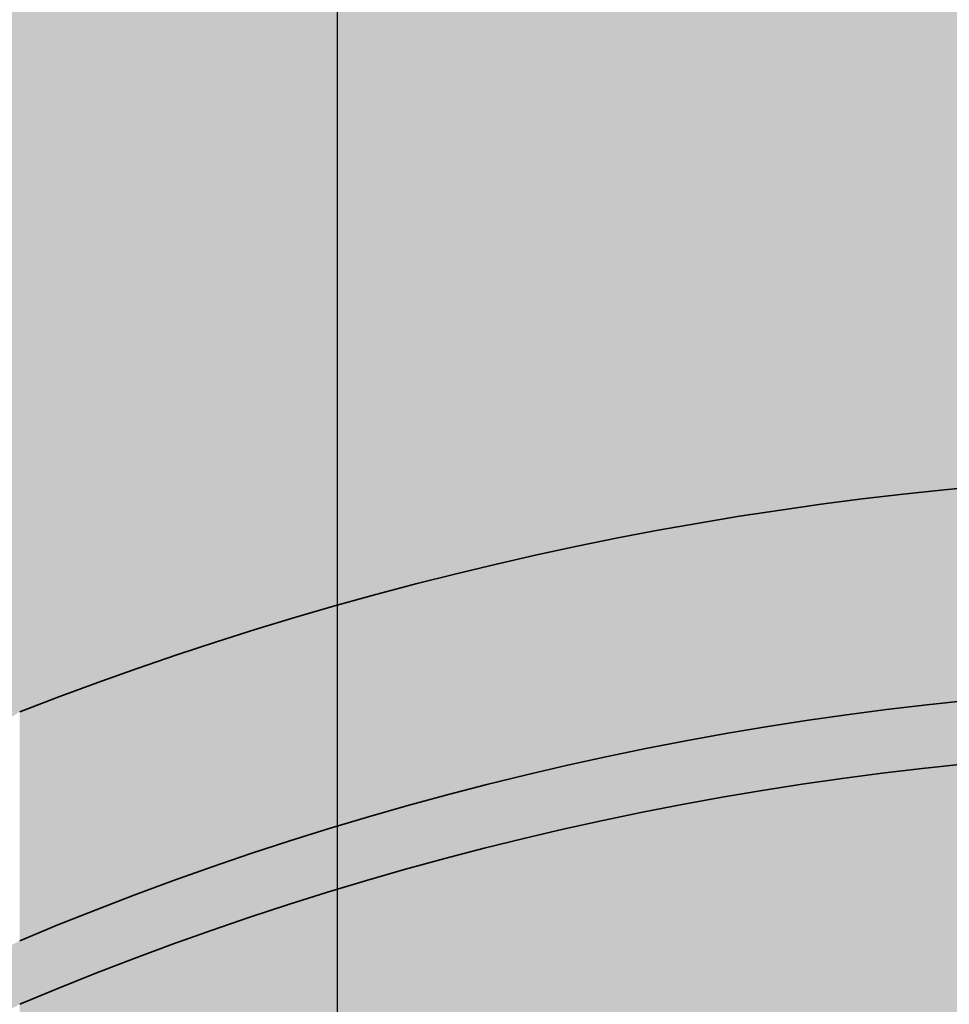
# Model space of a CAD drawing. Units: millimetres. Extents: x 130 to 1021, y 147 to 699.
# Tile 6 of 40: x 367 to 411, y 394 to 440. Entities that reach past the tile are written whole.
import ezdxf

# ---------------------------------------------------------------- set-up
doc = ezdxf.new("R2010")
doc.units = ezdxf.units.MM
doc.header["$MEASUREMENT"] = 0
for name, color, linetype, lineweight in [('A-ANNO-DIMS', 2, 'Continuous', 18), ('A-ELEV', 7, 'Continuous', 35), ('A-ELEV-PATT', 9, 'Continuous', 13)]:
    doc.layers.add(name, color=color, linetype=linetype, lineweight=lineweight)
doc.styles.get("Standard").update_dxf_attribs({"font": 'arial.ttf'})
doc.dimstyles.get("Standard").update_dxf_attribs({"dimtxt": 20, "dimasz": 10, "dimexe": 10, "dimexo": 10, "dimgap": 5, "dimtad": 0, "dimtih": 1, "dimtoh": 1, "dimdec": 0, "dimzin": 0, "dimdsep": 46, "dimtxsty": 'Standard', "dimcen": 5, "dimadec": 0, "dimazin": 0, "dimtfac": 1, "dimtdec": 0, "dimtofl": 0, "dimtmove": 0, "dimatfit": 3, "dimfxl": 1, "dimtolj": 1, "dimtzin": 0, "dimarcsym": 0})

# ---------------------------------------------------------------- blocks, each defined once
blk = doc.blocks.new('*D7')
at = {"layer": 'A-ANNO-DIMS', "color": 0, "lineweight": -2, "transparency": 16777216}
for p, q in [((399.374, 349.447), (413.374, 349.447)), ((423.374, 349.447), (433.374, 349.447)), ((389.374, 344.547), (389.374, 339.447)), ((423.374, 344.547), (423.374, 339.447))]:
    blk.add_line(p, q, dxfattribs=at)
at = {"layer": 'A-ANNO-DIMS', "color": 0, "transparency": 16777216}
for points in [[(399.374, 351.114), (399.374, 347.781), (389.374, 349.447)], [(413.374, 351.114), (413.374, 347.781), (423.374, 349.447)]]:
    blk.add_solid(points, dxfattribs=at)
at = {"layer": 'Defpoints', "color": 0, "transparency": 16777216}
for p in [(389.374, 354.547), (423.374, 354.547), (423.374, 349.447)]:
    blk.add_point(p, dxfattribs=at)
at = {"layer": 'A-ANNO-DIMS', "color": 0, "transparency": 16777216, "insert": (582.037, 349.447), "char_height": 20, "attachment_point": 5}
blk.add_mtext('\\A1;DOOR PANEL 34 TYP.', dxfattribs=at)
blk = doc.blocks.new('*D11')
at = {"layer": 'A-ANNO-DIMS', "color": 0, "lineweight": -2, "transparency": 16777216}
for p, q in [((737.374, 648.699), (737.374, 149.739)), ((299.374, 566.947), (299.374, 149.739)), ((309.374, 159.739), (490.857, 159.739)), ((727.374, 159.739), (545.891, 159.739))]:
    blk.add_line(p, q, dxfattribs=at)
at = {"layer": 'A-ANNO-DIMS', "color": 0, "transparency": 16777216}
for points in [[(309.374, 161.406), (309.374, 158.073), (299.374, 159.739)], [(727.374, 161.406), (727.374, 158.073), (737.374, 159.739)]]:
    blk.add_solid(points, dxfattribs=at)
at = {"layer": 'Defpoints', "color": 0, "transparency": 16777216}
for p in [(737.374, 658.699), (299.374, 576.947), (737.374, 159.739)]:
    blk.add_point(p, dxfattribs=at)
at = {"layer": 'A-ANNO-DIMS', "color": 0, "transparency": 16777216, "insert": (518.374, 159.739), "char_height": 20, "attachment_point": 5}
blk.add_mtext('\\A1;438', dxfattribs=at)
blk = doc.blocks.new('*D12')
at = {"layer": 'A-ANNO-DIMS', "color": 0, "lineweight": -2, "transparency": 16777216}
for p, q in [((477.374, 661.947), (265.074, 661.947)), ((275.074, 651.947), (275.074, 438.205)), ((275.074, 194.039), (275.074, 407.782)), ((357.163, 184.039), (265.074, 184.039))]:
    blk.add_line(p, q, dxfattribs=at)
at = {"layer": 'A-ANNO-DIMS', "color": 0, "transparency": 16777216}
for points in [[(273.407, 651.947), (276.74, 651.947), (275.074, 661.947)], [(273.407, 194.039), (276.74, 194.039), (275.074, 184.039)]]:
    blk.add_solid(points, dxfattribs=at)
at = {"layer": 'Defpoints', "color": 0, "transparency": 16777216}
for p in [(275.074, 661.947), (487.374, 661.947), (367.163, 184.039)]:
    blk.add_point(p, dxfattribs=at)
at = {"layer": 'A-ANNO-DIMS', "color": 0, "transparency": 16777216, "insert": (275.074, 422.993), "char_height": 20, "attachment_point": 5}
blk.add_mtext('\\A1;477.9', dxfattribs=at)
blk = doc.blocks.new('*D15')
at = {"layer": 'A-ANNO-DIMS', "color": 0, "lineweight": -2, "transparency": 16777216}
for p, q in [((327.374, 579.884), (327.374, 696.247)), ((357.941, 411.947), (357.941, 696.247)), ((337.374, 686.247), (347.941, 686.247)), ((357.941, 686.247), (367.941, 686.247))]:
    blk.add_line(p, q, dxfattribs=at)
at = {"layer": 'A-ANNO-DIMS', "color": 0, "transparency": 16777216}
for points in [[(337.374, 687.914), (337.374, 684.581), (327.374, 686.247)], [(347.941, 687.914), (347.941, 684.581), (357.941, 686.247)]]:
    blk.add_solid(points, dxfattribs=at)
at = {"layer": 'Defpoints', "color": 0, "transparency": 16777216}
for p in [(357.941, 686.247), (327.374, 569.884), (357.941, 401.947)]:
    blk.add_point(p, dxfattribs=at)
at = {"layer": 'A-ANNO-DIMS', "color": 0, "transparency": 16777216, "insert": (406.679, 686.247), "char_height": 20, "attachment_point": 5}
blk.add_mtext('\\A1;30.57', dxfattribs=at)
blk = doc.blocks.new('*D16')
at = {"layer": 'A-ANNO-DIMS', "color": 0, "lineweight": -2, "transparency": 16777216}
for p, q in [((357.941, 411.947), (357.941, 696.247)), ((363.922, 579.884), (363.922, 696.247)), ((347.941, 686.247), (337.941, 686.247)), ((373.922, 686.247), (383.922, 686.247))]:
    blk.add_line(p, q, dxfattribs=at)
at = {"layer": 'A-ANNO-DIMS', "color": 0, "transparency": 16777216}
for points in [[(347.941, 687.914), (347.941, 684.581), (357.941, 686.247)], [(373.922, 687.914), (373.922, 684.581), (363.922, 686.247)]]:
    blk.add_solid(points, dxfattribs=at)
at = {"layer": 'Defpoints', "color": 0, "transparency": 16777216}
for p in [(363.922, 686.247), (363.922, 569.884), (357.941, 401.947)]:
    blk.add_point(p, dxfattribs=at)
at = {"layer": 'A-ANNO-DIMS', "color": 0, "transparency": 16777216, "insert": (420.737, 686.247), "char_height": 20, "attachment_point": 5}
blk.add_mtext('\\A1;5.981', dxfattribs=at)
blk = doc.blocks.new('*D18')
at = {"layer": 'A-ANNO-DIMS', "color": 0, "lineweight": -2, "transparency": 16777216}
for p, q in [((375.85, 490.216), (375.85, 696.247)), ((382.374, 388.947), (382.374, 696.247)), ((365.85, 686.247), (355.85, 686.247)), ((392.374, 686.247), (402.374, 686.247))]:
    blk.add_line(p, q, dxfattribs=at)
at = {"layer": 'A-ANNO-DIMS', "color": 0, "transparency": 16777216}
for points in [[(365.85, 687.914), (365.85, 684.581), (375.85, 686.247)], [(392.374, 687.914), (392.374, 684.581), (382.374, 686.247)]]:
    blk.add_solid(points, dxfattribs=at)
at = {"layer": 'Defpoints', "color": 0, "transparency": 16777216}
for p in [(382.374, 686.247), (375.85, 480.216), (382.374, 378.947)]:
    blk.add_point(p, dxfattribs=at)
at = {"layer": 'A-ANNO-DIMS', "color": 0, "transparency": 16777216, "insert": (441.132, 686.247), "char_height": 20, "attachment_point": 5}
blk.add_mtext('\\A1;6.524', dxfattribs=at)
blk = doc.blocks.new('*D19')
at = {"layer": 'A-ANNO-DIMS', "color": 0, "lineweight": -2, "transparency": 16777216}
for p, q in [((382.374, 388.947), (382.374, 696.247)), ((414.652, 510.881), (414.652, 696.247)), ((392.374, 686.247), (404.652, 686.247)), ((414.652, 686.247), (424.652, 686.247))]:
    blk.add_line(p, q, dxfattribs=at)
at = {"layer": 'A-ANNO-DIMS', "color": 0, "transparency": 16777216}
for points in [[(392.374, 687.914), (392.374, 684.581), (382.374, 686.247)], [(404.652, 687.914), (404.652, 684.581), (414.652, 686.247)]]:
    blk.add_solid(points, dxfattribs=at)
at = {"layer": 'Defpoints', "color": 0, "transparency": 16777216}
for p in [(414.652, 686.247), (414.652, 500.881), (382.374, 378.947)]:
    blk.add_point(p, dxfattribs=at)
at = {"layer": 'A-ANNO-DIMS', "color": 0, "transparency": 16777216, "insert": (463.411, 686.247), "char_height": 20, "attachment_point": 5}
blk.add_mtext('\\A1;32.28', dxfattribs=at)
blk = doc.blocks.new('*D20')
at = {"layer": 'A-ANNO-DIMS', "color": 0, "lineweight": -2, "transparency": 16777216}
for p, q in [((414.652, 510.881), (414.652, 696.247)), ((432.374, 388.947), (432.374, 696.247)), ((404.652, 686.247), (394.652, 686.247)), ((442.374, 686.247), (452.374, 686.247))]:
    blk.add_line(p, q, dxfattribs=at)
at = {"layer": 'A-ANNO-DIMS', "color": 0, "transparency": 16777216}
for points in [[(404.652, 687.914), (404.652, 684.581), (414.652, 686.247)], [(442.374, 687.914), (442.374, 684.581), (432.374, 686.247)]]:
    blk.add_solid(points, dxfattribs=at)
at = {"layer": 'Defpoints', "color": 0, "transparency": 16777216}
for p in [(432.374, 686.247), (414.652, 500.881), (432.374, 378.947)]:
    blk.add_point(p, dxfattribs=at)
at = {"layer": 'A-ANNO-DIMS', "color": 0, "transparency": 16777216, "insert": (490.075, 686.247), "char_height": 20, "attachment_point": 5}
blk.add_mtext('\\A1;17.72', dxfattribs=at)
blk = doc.blocks.new('*D64')
at = {"layer": 'A-ANNO-DIMS', "color": 0, "lineweight": -2, "transparency": 16777216}
for p, q in [((502.049, 450.926), (502.049, 460.926)), ((497.049, 455.926), (507.049, 455.926)), ((363.96, 263.061), (409.922, 327.255)), ((353.96, 263.061), (363.96, 263.061))]:
    blk.add_line(p, q, dxfattribs=at)
at = {"layer": 'A-ANNO-DIMS', "color": 0, "transparency": 16777216}
blk.add_solid([(408.567, 328.225), (411.277, 326.284), (415.743, 335.385)], dxfattribs=at)
at = {"layer": 'Defpoints', "color": 0, "transparency": 16777216}
for p in [(502.049, 455.926), (415.743, 335.385)]:
    blk.add_point(p, dxfattribs=at)
at = {"layer": 'A-ANNO-DIMS', "color": 0, "transparency": 16777216, "insert": (297.8, 263.061), "char_height": 20, "attachment_point": 5}
blk.add_mtext('\\A1;R148.25', dxfattribs=at)
blk = doc.blocks.new('*D66')
at = {"layer": 'A-ANNO-DIMS', "color": 0, "lineweight": -2, "transparency": 16777216}
for p, q in [((341.579, 557.194), (351.579, 557.194)), ((351.579, 557.194), (376.947, 478.135)), ((427.374, 315.978), (427.374, 325.978)), ((422.374, 320.978), (432.374, 320.978))]:
    blk.add_line(p, q, dxfattribs=at)
at = {"layer": 'A-ANNO-DIMS', "color": 0, "transparency": 16777216}
blk.add_solid([(378.534, 478.644), (375.36, 477.626), (380.002, 468.613)], dxfattribs=at)
at = {"layer": 'Defpoints', "color": 0, "transparency": 16777216}
for p in [(380.002, 468.613), (427.374, 320.978)]:
    blk.add_point(p, dxfattribs=at)
at = {"layer": 'A-ANNO-DIMS', "color": 0, "transparency": 16777216, "insert": (263.53, 557.194), "char_height": 20, "attachment_point": 5}
blk.add_mtext('\\A1;4X R155.05', dxfattribs=at)
blk = doc.blocks.new('*D68')
at = {"layer": 'A-ANNO-DIMS', "color": 0, "lineweight": -2, "transparency": 16777216}
for p, q in [((361.841, 579.756), (371.841, 579.756)), ((371.841, 579.756), (392.167, 506.693)), ((433.191, 354.23), (433.191, 364.23)), ((428.191, 359.23), (438.191, 359.23))]:
    blk.add_line(p, q, dxfattribs=at)
at = {"layer": 'A-ANNO-DIMS', "color": 0, "transparency": 16777216}
blk.add_solid([(393.773, 507.14), (390.561, 506.246), (394.847, 497.059)], dxfattribs=at)
at = {"layer": 'Defpoints', "color": 0, "transparency": 16777216}
for p in [(394.847, 497.059), (433.191, 359.23)]:
    blk.add_point(p, dxfattribs=at)
at = {"layer": 'A-ANNO-DIMS', "color": 0, "transparency": 16777216, "insert": (305.764, 579.756), "char_height": 20, "attachment_point": 5}
blk.add_mtext('\\A1;R143.06', dxfattribs=at)
blk = doc.blocks.new('*D70')
at = {"layer": 'A-ANNO-DIMS', "color": 0, "lineweight": -2, "transparency": 16777216}
for p, q in [((370.141, 588.4), (380.141, 588.4)), ((380.141, 588.4), (397.473, 517.008)), ((432.65, 367.109), (432.65, 377.109)), ((427.65, 372.109), (437.65, 372.109))]:
    blk.add_line(p, q, dxfattribs=at)
at = {"layer": 'A-ANNO-DIMS', "color": 0, "transparency": 16777216}
blk.add_solid([(399.093, 517.402), (395.854, 516.615), (399.832, 507.291)], dxfattribs=at)
at = {"layer": 'Defpoints', "color": 0, "transparency": 16777216}
for p in [(399.832, 507.291), (432.65, 372.109)]:
    blk.add_point(p, dxfattribs=at)
at = {"layer": 'A-ANNO-DIMS', "color": 0, "transparency": 16777216, "insert": (323.757, 588.4), "char_height": 20, "attachment_point": 5}
blk.add_mtext('\\A1;R139.1', dxfattribs=at)
blk = doc.blocks.new('*D73')
at = {"layer": 'A-ANNO-DIMS', "color": 0, "lineweight": -2, "transparency": 16777216}
for p, q in [((402.678, 571.448), (412.678, 571.448)), ((412.678, 571.448), (419.051, 502.166)), ((432.115, 355.142), (432.115, 365.142)), ((427.115, 360.142), (437.115, 360.142))]:
    blk.add_line(p, q, dxfattribs=at)
at = {"layer": 'A-ANNO-DIMS', "color": 0, "transparency": 16777216}
blk.add_solid([(420.711, 502.319), (417.391, 502.014), (419.967, 492.208)], dxfattribs=at)
at = {"layer": 'Defpoints', "color": 0, "transparency": 16777216}
for p in [(419.967, 492.208), (432.115, 360.142)]:
    blk.add_point(p, dxfattribs=at)
at = {"layer": 'A-ANNO-DIMS', "color": 0, "transparency": 16777216, "insert": (346.696, 571.448), "char_height": 20, "attachment_point": 5}
blk.add_mtext('\\A1;R132.62', dxfattribs=at)

msp = doc.modelspace()

# ---------------------------------------------------------------- hatches: boundary and pattern name
at = {"layer": 'A-ELEV-PATT'}
h = msp.add_hatch(color=256, dxfattribs=at)
h.dxf.hatch_style = 1
h.paths.add_polyline_path([(737.3738, 658.6988, 0.0135961), (632.4019, 661.9473), (607.3738, 661.9473), (487.3738, 661.9473), (487.3738, 649.9473), (607.3738, 649.9473), (632.3794, 649.9473, -0.0136841), (737.3738, 646.6784)])
h.paths.add_polyline_path([(732.3738, 643.9599, 0.0130529), (632.3738, 646.9473), (607.3738, 646.9473), (487.3738, 646.9473), (487.3738, 596.9473), (632.3738, 596.9473, -0.0130529), (732.3738, 593.9599)])
h.paths.add_polyline_path([(737.3738, 593.6732, 0.0137063), (632.3738, 596.9473), (487.3738, 596.9473), (487.3738, 586.9473), (632.355, 586.9473, -0.0137808), (737.3738, 583.6559)])
h.paths.add_polyline_path([(447.3738, 646.9473), (307.3738, 646.9473), (302.3738, 646.9473), (302.3738, 634.9473), (447.3738, 634.9473)])
h.paths.add_polyline_path([(447.3738, 631.9473), (307.3738, 631.9473), (307.3738, 586.9473), (447.3738, 586.9473)])
h.paths.add_polyline_path([(447.3738, 586.9473), (307.3738, 586.9473), (302.3738, 586.9473), (302.3738, 576.9473), (447.3738, 576.9473)])
h.paths.add_polyline_path([(447.3738, 573.9473), (367.3738, 573.9473), (367.3738, 539.9473), (447.3738, 539.9473)])
h.paths.add_polyline_path([(447.3738, 537.9473), (367.3738, 537.9473), (367.3738, 507.9473), (400.392, 507.4253, -0.001728), (401.3281, 507.6451, -0.5220025), (425.6117, 511.0391, -0.0391849), (447.3738, 510.4359), (447.3738, 510.7883)])
h.paths.add_polyline_path([(394.7238, 505.9473), (367.3738, 505.9473), (367.3738, 476.9473, -0.0146512), (375.8501, 480.2159), (376.1506, 499.2266, -0.0355419)])
h.paths.add_polyline_path([(632.3738, 583.9473), (552.3738, 583.9473), (552.3738, 550.9473), (632.3738, 550.9473)])
h.paths.add_polyline_path([(632.3738, 548.9473), (552.3738, 548.9473), (552.3738, 515.9473), (632.3738, 515.9473)])
h.paths.add_polyline_path([(632.3738, 513.9473), (552.3738, 513.9473), (552.3738, 476.9473), (632.3738, 476.9473)])
h.paths.add_polyline_path([(737.3738, 473.6903, 0.0136326), (632.3926, 476.9473), (552.3738, 476.9473), (487.3738, 476.9473), (487.3738, 466.9473), (632.3738, 466.9473, -0.0137063), (737.3738, 463.6732)])
h.paths.add_polyline_path([(732.3738, 460.9552, 0.0130741), (632.3681, 463.9473), (487.3738, 463.9473), (487.3738, 407.735, -0.0032286), (489.3544, 406.9473), (632.3926, 406.9473, -0.0129826), (732.3738, 403.9755)])
h.paths.add_polyline_path([(487.3738, 463.9473, 0.20133), (367.3738, 463.9473), (367.3738, 407.735, -0.1882031), (487.3738, 407.735)])
h.paths.add_polyline_path([(367.3738, 476.9473), (367.3738, 466.9473, -0.2013309), (487.3738, 466.9473), (487.3738, 476.9473, 0.20133)])
h.paths.add_polyline_path([(367.3738, 463.9473), (307.3738, 463.9473), (307.3738, 401.9473), (357.9413, 401.9473), (367.3738, 407.735)])
h.paths.add_polyline_path([(367.3738, 476.9473), (302.3738, 476.9473), (302.3738, 466.9473), (367.3738, 466.9473)])
h.paths.add_polyline_path([(632.8184, 366.9453), (552.3738, 366.9453), (552.3738, 393.9473), (632.8184, 393.9473)])
h.paths.add_polyline_path([(632.8184, 357.2114), (632.8184, 363.9453), (552.3738, 363.9453), (552.3738, 357.2114), (552.3738, 336.9453), (632.8184, 336.9453)])
h.paths.add_polyline_path([(632.8184, 333.9453), (552.3738, 333.9453), (552.3738, 306.9453), (632.8184, 306.9453)])
h.paths.add_polyline_path([(632.8184, 303.9453), (552.3738, 303.9453), (552.3738, 273.9473), (632.355, 273.9473, 0.0000608), (632.8184, 273.9491)])
h.paths.add_polyline_path([(737.3738, 403.6903, 0.0136326), (632.3926, 406.9473), (489.3544, 406.9473, 0.1915481), (367.3738, 407.735), (367.3738, 396.9473, -0.2013309), (487.3738, 396.9473), (632.3738, 396.9473, -0.0137063), (737.3738, 393.6732)])
h.paths.add_polyline_path([(357.9413, 401.9473), (307.3738, 401.9473), (307.3738, 391.9473), (357.9413, 391.9473)])
h.paths.add_polyline_path([(357.9413, 357.2114), (357.9413, 388.9473), (307.3738, 388.9473), (307.3738, 357.2114), (307.3738, 273.9473), (357.9413, 273.9473)])
h.paths.add_polyline_path([(732.3738, 263.93, -0.0130317), (632.3794, 260.9473), (466.7667, 260.9473), (466.7667, 240.9473), (469.8406, 236.978), (469.8406, 221.978), (472.9145, 218.0087), (472.9145, 213.9473), (607.3738, 213.9473), (732.3738, 213.9473)])
h.paths.add_polyline_path([(732.3738, 290.889), (722.479, 290.889), (722.479, 301.889), (732.3738, 301.889), (732.3738, 305.889), (722.479, 305.889), (722.479, 316.889), (732.3738, 316.889), (732.3738, 320.889), (722.479, 320.889), (722.479, 331.889), (732.3738, 331.889), (732.3738, 335.889), (722.479, 335.889), (722.479, 346.889), (732.3738, 346.889), (732.3738, 350.889), (722.479, 350.889), (722.479, 361.889), (732.3738, 361.889), (732.3738, 365.889), (722.479, 365.889), (722.479, 376.889), (732.3738, 376.889), (732.3738, 380.889), (722.479, 380.889), (722.479, 391.4848, 0.0005233), (718.479, 391.6843), (718.479, 380.889), (707.479, 380.889), (707.479, 392.1896, 0.0005231), (703.479, 392.3576), (703.479, 380.889), (692.479, 380.889), (692.479, 392.7765, 0.0005229), (688.479, 392.9131), (688.479, 380.889), (677.479, 380.889), (677.479, 393.2456, 0.0005228), (673.479, 393.3508), (673.479, 380.889), (662.479, 380.889), (662.479, 393.597, 0.0005227), (658.479, 393.6709), (658.479, 380.889), (647.479, 380.889), (647.479, 393.8308, 0.0005226), (643.479, 393.8732), (643.479, 380.889), (632.8184, 380.889), (632.8184, 376.889), (643.479, 376.889), (643.479, 365.889), (632.8184, 365.889), (632.8184, 361.889), (643.479, 361.889), (643.479, 350.889), (632.8184, 350.889), (632.8184, 346.889), (643.479, 346.889), (643.479, 335.889), (632.8184, 335.889), (632.8184, 331.889), (643.479, 331.889), (643.479, 320.889), (632.8184, 320.889), (632.8184, 316.889), (643.479, 316.889), (643.479, 305.889), (632.8184, 305.889), (632.8184, 301.889), (643.479, 301.889), (643.479, 290.889), (632.8184, 290.889), (632.8184, 286.889), (643.479, 286.889), (643.479, 274.0217, 0.0005246), (647.479, 274.0643), (647.479, 286.889), (658.479, 286.889), (658.479, 274.2248, 0.0005246), (662.479, 274.2989), (662.479, 286.889), (673.479, 286.889), (673.479, 274.546, 0.0005247), (677.479, 274.6516), (677.479, 286.889), (688.479, 286.889), (688.479, 274.9853, 0.0005248), (692.479, 275.1224), (692.479, 286.889), (703.479, 286.889), (703.479, 275.5429, 0.000525), (707.479, 275.7115), (707.479, 286.889), (718.479, 286.889), (718.479, 276.2187, 0.0005252), (722.479, 276.4189), (722.479, 286.889), (732.3738, 286.889)])
h.paths.add_polyline_path([(718.479, 290.889), (707.479, 290.889), (707.479, 301.889), (718.479, 301.889)], flags=16)
h.paths.add_polyline_path([(703.479, 290.889), (692.479, 290.889), (692.479, 301.889), (703.479, 301.889)], flags=16)
h.paths.add_polyline_path([(718.479, 305.889), (707.479, 305.889), (707.479, 316.889), (718.479, 316.889)], flags=16)
h.paths.add_polyline_path([(703.479, 305.889), (692.479, 305.889), (692.479, 316.889), (703.479, 316.889)], flags=16)
h.paths.add_polyline_path([(688.479, 290.889), (677.479, 290.889), (677.479, 301.889), (688.479, 301.889)], flags=16)
h.paths.add_polyline_path([(718.479, 320.889), (707.479, 320.889), (707.479, 331.889), (718.479, 331.889)], flags=16)
h.paths.add_polyline_path([(688.479, 305.889), (677.479, 305.889), (677.479, 316.889), (688.479, 316.889)], flags=16)
h.paths.add_polyline_path([(703.479, 320.889), (692.479, 320.889), (692.479, 331.889), (703.479, 331.889)], flags=16)
h.paths.add_polyline_path([(688.479, 320.889), (677.479, 320.889), (677.479, 331.889), (688.479, 331.889)], flags=16)
h.paths.add_polyline_path([(673.479, 290.889), (662.479, 290.889), (662.479, 301.889), (673.479, 301.889)], flags=16)
h.paths.add_polyline_path([(718.479, 335.889), (707.479, 335.889), (707.479, 346.889), (718.479, 346.889)], flags=16)
h.paths.add_polyline_path([(673.479, 305.889), (662.479, 305.889), (662.479, 316.889), (673.479, 316.889)], flags=16)
h.paths.add_polyline_path([(703.479, 335.889), (692.479, 335.889), (692.479, 346.889), (703.479, 346.889)], flags=16)
h.paths.add_polyline_path([(673.479, 320.889), (662.479, 320.889), (662.479, 331.889), (673.479, 331.889)], flags=16)
h.paths.add_polyline_path([(688.479, 335.889), (677.479, 335.889), (677.479, 346.889), (688.479, 346.889)], flags=16)
h.paths.add_polyline_path([(658.479, 290.889), (647.479, 290.889), (647.479, 301.889), (658.479, 301.889)], flags=16)
h.paths.add_polyline_path([(718.479, 350.889), (707.479, 350.889), (707.479, 361.889), (718.479, 361.889)], flags=16)
h.paths.add_polyline_path([(658.479, 305.889), (647.479, 305.889), (647.479, 316.889), (658.479, 316.889)], flags=16)
h.paths.add_polyline_path([(703.479, 350.889), (692.479, 350.889), (692.479, 361.889), (703.479, 361.889)], flags=16)
h.paths.add_polyline_path([(673.479, 335.889), (662.479, 335.889), (662.479, 346.889), (673.479, 346.889)], flags=16)
h.paths.add_polyline_path([(658.479, 320.889), (647.479, 320.889), (647.479, 331.889), (658.479, 331.889)], flags=16)
h.paths.add_polyline_path([(688.479, 350.889), (677.479, 350.889), (677.479, 361.889), (688.479, 361.889)], flags=16)
h.paths.add_polyline_path([(718.479, 365.889), (707.479, 365.889), (707.479, 376.889), (718.479, 376.889)], flags=16)
h.paths.add_polyline_path([(658.479, 335.889), (647.479, 335.889), (647.479, 346.889), (658.479, 346.889)], flags=16)
h.paths.add_polyline_path([(673.479, 350.889), (662.479, 350.889), (662.479, 361.889), (673.479, 361.889)], flags=16)
h.paths.add_polyline_path([(703.479, 365.889), (692.479, 365.889), (692.479, 376.889), (703.479, 376.889)], flags=16)
h.paths.add_polyline_path([(688.479, 365.889), (677.479, 365.889), (677.479, 376.889), (688.479, 376.889)], flags=16)
h.paths.add_polyline_path([(658.479, 350.889), (647.479, 350.889), (647.479, 361.889), (658.479, 361.889)], flags=16)
h.paths.add_polyline_path([(673.479, 365.889), (662.479, 365.889), (662.479, 376.889), (673.479, 376.889)], flags=16)
h.paths.add_polyline_path([(658.479, 365.889), (647.479, 365.889), (647.479, 376.889), (658.479, 376.889)], flags=16)
h.paths.add_polyline_path([(732.3738, 503.9786), (722.3392, 503.9786), (722.3392, 514.9786), (732.3738, 514.9786), (732.3738, 518.9786), (722.3392, 518.9786), (722.3392, 529.9786), (732.3738, 529.9786), (732.3738, 533.9786), (722.3392, 533.9786), (722.3392, 544.9786), (732.3738, 544.9786), (732.3738, 546.9473), (732.3738, 548.9786), (722.3392, 548.9786), (722.3392, 559.9786), (732.3738, 559.9786), (732.3738, 563.9786), (722.3392, 563.9786), (722.3392, 574.9786), (732.3738, 574.9786), (732.3738, 578.9786), (722.3392, 578.9786), (722.3392, 581.4789, 0.000526), (718.3392, 581.6791), (718.3392, 578.9786), (707.3392, 578.9786), (707.3392, 582.1863, 0.0005258), (703.3392, 582.355), (703.3392, 578.9786), (692.3392, 578.9786), (692.3392, 582.7752, 0.0005257), (688.3392, 582.9123), (688.3392, 578.9786), (677.3392, 578.9786), (677.3392, 583.2457, 0.0005255), (673.3392, 583.3512), (673.3392, 578.9786), (662.3392, 578.9786), (662.3392, 583.5978, 0.0005254), (658.3392, 583.6718), (658.3392, 578.9786), (647.3392, 578.9786), (647.3392, 583.8317, 0.0005254), (643.3392, 583.8741), (643.3392, 578.9786), (632.3738, 578.9786), (632.3738, 574.9786), (643.3392, 574.9786), (643.3392, 563.9786), (632.3738, 563.9786), (632.3738, 559.9786), (643.3392, 559.9786), (643.3392, 548.9786), (632.3738, 548.9786), (632.3738, 544.9786), (643.3392, 544.9786), (643.3392, 533.9786), (632.3738, 533.9786), (632.3738, 529.9786), (643.3392, 529.9786), (643.3392, 518.9786), (632.3738, 518.9786), (632.3738, 515.9473), (632.3738, 514.9786), (643.3392, 514.9786), (643.3392, 503.9786), (632.3738, 503.9786), (632.3738, 499.9786), (643.3392, 499.9786), (643.3392, 488.9786), (632.3738, 488.9786), (632.3738, 484.9786), (643.3392, 484.9786), (643.3392, 476.8751, -0.0005191), (647.3392, 476.8332), (647.3392, 484.9786), (658.3392, 484.9786), (658.3392, 476.6752, -0.0005192), (662.3392, 476.6022), (662.3392, 484.9786), (673.3392, 484.9786), (673.3392, 476.3585, -0.0005193), (677.3392, 476.2543), (677.3392, 484.9786), (688.3392, 484.9786), (688.3392, 475.9248, -0.0005194), (692.3392, 475.7894), (692.3392, 484.9786), (703.3392, 484.9786), (703.3392, 475.3741, -0.0005195), (707.3392, 475.2075), (707.3392, 484.9786), (718.3392, 484.9786), (718.3392, 474.7064, -0.0005197), (722.3392, 474.5086), (722.3392, 484.9786), (732.3738, 484.9786), (732.3738, 488.9786), (722.3392, 488.9786), (722.3392, 499.9786), (732.3738, 499.9786)])
h.paths.add_polyline_path([(718.3392, 503.9786), (707.3392, 503.9786), (707.3392, 514.9786), (718.3392, 514.9786)], flags=16)
h.paths.add_polyline_path([(718.3392, 499.9786), (718.3392, 488.9786), (707.3392, 488.9786), (707.3392, 499.9786)], flags=16)
h.paths.add_polyline_path([(718.3392, 518.9786), (707.3392, 518.9786), (707.3392, 529.9786), (718.3392, 529.9786)], flags=16)
h.paths.add_polyline_path([(703.3392, 503.9786), (692.3392, 503.9786), (692.3392, 514.9786), (703.3392, 514.9786)], flags=16)
h.paths.add_polyline_path([(703.3392, 499.9786), (703.3392, 488.9786), (692.3392, 488.9786), (692.3392, 499.9786)], flags=16)
h.paths.add_polyline_path([(703.3392, 518.9786), (692.3392, 518.9786), (692.3392, 529.9786), (703.3392, 529.9786)], flags=16)
h.paths.add_polyline_path([(718.3392, 533.9786), (707.3392, 533.9786), (707.3392, 544.9786), (718.3392, 544.9786)], flags=16)
h.paths.add_polyline_path([(688.3392, 503.9786), (677.3392, 503.9786), (677.3392, 514.9786), (688.3392, 514.9786)], flags=16)
h.paths.add_polyline_path([(688.3392, 499.9786), (688.3392, 488.9786), (677.3392, 488.9786), (677.3392, 499.9786)], flags=16)
h.paths.add_polyline_path([(703.3392, 533.9786), (692.3392, 533.9786), (692.3392, 544.9786), (703.3392, 544.9786)], flags=16)
h.paths.add_polyline_path([(688.3392, 518.9786), (677.3392, 518.9786), (677.3392, 529.9786), (688.3392, 529.9786)], flags=16)
h.paths.add_polyline_path([(688.3392, 533.9786), (677.3392, 533.9786), (677.3392, 544.9786), (688.3392, 544.9786)], flags=16)
h.paths.add_polyline_path([(718.3392, 548.9786), (707.3392, 548.9786), (707.3392, 559.9786), (718.3392, 559.9786)], flags=16)
h.paths.add_polyline_path([(673.3392, 503.9786), (662.3392, 503.9786), (662.3392, 514.9786), (673.3392, 514.9786)], flags=16)
h.paths.add_polyline_path([(673.3392, 499.9786), (673.3392, 488.9786), (662.3392, 488.9786), (662.3392, 499.9786)], flags=16)
h.paths.add_polyline_path([(703.3392, 548.9786), (692.3392, 548.9786), (692.3392, 559.9786), (703.3392, 559.9786)], flags=16)
h.paths.add_polyline_path([(673.3392, 518.9786), (662.3392, 518.9786), (662.3392, 529.9786), (673.3392, 529.9786)], flags=16)
h.paths.add_polyline_path([(688.3392, 548.9786), (677.3392, 548.9786), (677.3392, 559.9786), (688.3392, 559.9786)], flags=16)
h.paths.add_polyline_path([(673.3392, 533.9786), (662.3392, 533.9786), (662.3392, 544.9786), (673.3392, 544.9786)], flags=16)
h.paths.add_polyline_path([(718.3392, 563.9786), (707.3392, 563.9786), (707.3392, 574.9786), (718.3392, 574.9786)], flags=16)
h.paths.add_polyline_path([(658.3392, 503.9786), (647.3392, 503.9786), (647.3392, 514.9786), (658.3392, 514.9786)], flags=16)
h.paths.add_polyline_path([(658.3392, 499.9786), (658.3392, 488.9786), (647.3392, 488.9786), (647.3392, 499.9786)], flags=16)
h.paths.add_polyline_path([(703.3392, 563.9786), (692.3392, 563.9786), (692.3392, 574.9786), (703.3392, 574.9786)], flags=16)
h.paths.add_polyline_path([(658.3392, 518.9786), (647.3392, 518.9786), (647.3392, 529.9786), (658.3392, 529.9786)], flags=16)
h.paths.add_polyline_path([(673.3392, 548.9786), (662.3392, 548.9786), (662.3392, 559.9786), (673.3392, 559.9786)], flags=16)
h.paths.add_polyline_path([(688.3392, 563.9786), (677.3392, 563.9786), (677.3392, 574.9786), (688.3392, 574.9786)], flags=16)
h.paths.add_polyline_path([(658.3392, 533.9786), (647.3392, 533.9786), (647.3392, 544.9786), (658.3392, 544.9786)], flags=16)
h.paths.add_polyline_path([(673.3392, 563.9786), (662.3392, 563.9786), (662.3392, 574.9786), (673.3392, 574.9786)], flags=16)
h.paths.add_polyline_path([(658.3392, 548.9786), (647.3392, 548.9786), (647.3392, 559.9786), (658.3392, 559.9786)], flags=16)
h.paths.add_polyline_path([(658.3392, 563.9786), (647.3392, 563.9786), (647.3392, 574.9786), (658.3392, 574.9786)], flags=16)
h = msp.add_hatch(color=256, dxfattribs=at)
h.dxf.hatch_style = 1
h.paths.add_polyline_path([(447.3738, 576.9473), (302.3738, 576.9473), (302.3738, 573.9473), (447.3738, 573.9473)])
h.paths.add_polyline_path([(487.3738, 583.9473), (487.3738, 586.9473), (447.3738, 576.9473), (447.3738, 573.9473)])
h.paths.add_polyline_path([(632.355, 586.9473), (487.3738, 586.9473), (487.3738, 583.9473), (632.3738, 583.9473), (632.3738, 583.9472, -0.0138), (737.3738, 580.6507), (737.3738, 583.6559, 0.0137808)])
h.paths.add_polyline_path([(367.3738, 466.9473), (302.3738, 466.9473), (302.3738, 463.9473), (367.3738, 463.9473)])
h.paths.add_polyline_path([(487.3738, 463.9473), (487.3738, 466.9473, 0.2013309), (367.3738, 466.9473), (367.3738, 463.9473, -0.20133)])
h.paths.add_polyline_path([(632.3738, 466.9473), (487.3738, 466.9473), (487.3738, 463.9473), (632.3681, 463.9473, -0.0137285), (737.3738, 460.6681), (737.3738, 463.6732, 0.0137063)])
h.paths.add_polyline_path([(632.3738, 396.9473), (487.3738, 396.9473, 0.2013309), (367.3738, 396.9473), (367.3738, 393.9473, -0.2023717), (486.7667, 393.9473), (632.3681, 393.9473, -0.0137285), (737.3738, 390.6681), (737.3738, 393.6732, 0.0137063)])
h.paths.add_polyline_path([(357.9413, 391.9473), (307.3738, 391.9473), (307.3738, 388.9473), (357.9413, 388.9473)])
h.paths.add_polyline_path([(367.3738, 393.9473), (367.3738, 396.9473), (357.9413, 391.924), (357.9413, 388.9473), (358.058, 388.9473)])
h.paths.add_polyline_path([(737.3738, 264.2162), (737.3738, 267.2214, -0.0137063), (632.3738, 263.9473), (463.7667, 263.9473), (466.7667, 260.9473), (632.3794, 260.9473, 0.0136841)])
h.paths.add_polyline_path([(463.7667, 263.9473), (447.3738, 263.9473), (450.3738, 260.9473), (466.7667, 260.9473)])
h.paths.add_polyline_path([(447.3738, 263.9473), (432.3738, 263.9473), (432.3738, 260.9473), (450.3738, 260.9473)])
h.paths.add_polyline_path([(382.3738, 263.9473), (357.9413, 263.9473), (357.9413, 260.9473), (382.3738, 260.9473)])
h.paths.add_polyline_path([(357.9413, 263.9473), (307.3738, 263.9473), (307.3738, 260.9473), (357.9413, 260.9473)])
h = msp.add_hatch(color=256, dxfattribs=at)
h.dxf.hatch_style = 1
h.paths.add_polyline_path([(363.922, 569.884), (327.3738, 569.884), (327.3738, 557.9168), (363.922, 557.9168)])
h.paths.add_polyline_path([(547.7773, 577.3739), (502.3738, 577.3739), (502.3738, 566.2111), (547.7773, 566.2111)])
h.paths.add_polyline_path([(544.6354, 386.2639), (486.7667, 386.2639), (486.7667, 377.43), (544.6354, 377.43)])
h.paths.add_polyline_path([(496.0546, 377.43), (486.7667, 377.43), (486.7667, 370.4028)])
h.paths.add_polyline_path([(447.3738, 393.9473), (367.3738, 393.9473, 0.0500478), (382.3738, 368.424), (382.3738, 378.9473), (432.3738, 378.9473), (432.3738, 325.067, 0.0278945), (447.3738, 318.1243), (447.3738, 357.2114)])
h.paths.add_polyline_path([(463.5608, 388.6449), (450.8779, 388.6449), (450.8779, 363.0915), (463.5608, 363.0915)])
h.paths.add_polyline_path([(463.5608, 360.0915), (450.8779, 360.0915), (450.8779, 334.5915), (463.5608, 334.5915)])
h.paths.add_polyline_path([(463.5608, 331.5915), (450.8779, 331.5915), (450.8779, 316.785, 0.0224513), (463.5608, 312.7571)])
msp.add_hatch(color=256, dxfattribs=at).paths.add_polyline_path([(367.3738, 393.9473), (486.7667, 393.9473, 0.2023717)])
h = msp.add_hatch(color=256, dxfattribs=at)
h.dxf.hatch_style = 1
h.paths.add_polyline_path([(382.3738, 368.424, -0.0500478), (367.3738, 393.9473), (367.3738, 357.2114), (367.3738, 273.9473), (382.3738, 273.9473)])
h.paths.add_polyline_path([(432.3738, 273.9473), (447.3738, 273.9473), (447.3738, 318.1243, -0.0278945), (432.3738, 325.067)])
h.paths.add_polyline_path([(463.5608, 306.0915), (463.5608, 312.7571, -0.0224513), (450.8779, 316.785), (450.8779, 306.0915)])
h.paths.add_polyline_path([(450.8779, 303.0915), (450.8779, 277.5915), (463.5608, 277.5915), (463.5608, 303.0915)])

# ---------------------------------------------------------------- linework, layer by layer
at = {"layer": 'A-ELEV'}
for centre, radius, start, end in [((427.3738, 253.9788), 165.0484, 67.942927, 111.31713), ((427.3738, 253.9788), 155.0484, 67.233534, 112.766466), ((427.0702, 252.4956), 153.5326, 67.118929, 112.881071)]:
    msp.add_arc(centre, radius, start, end, dxfattribs=at)

# ---------------------------------------------------------------- dimensions: what is measured, and where the dimension line sits
at = {"layer": 'A-ANNO-DIMS'}
for base, p1, p2, override, picture, middle in [((357.9413, 686.2473), (327.3738, 569.884), (357.9413, 401.9473), {"dimdec": 2, "dimlfac": 1, "dimrnd": 0, "dimzin": 0, "dimdsep": 46, "dimlunit": 2}, '*D15', (406.6794, 686.2473)), ((363.922, 686.2473), (357.9413, 401.9473), (363.922, 569.884), {"dimdec": 3, "dimlfac": 1, "dimrnd": 0, "dimzin": 0, "dimdsep": 46, "dimlunit": 2}, '*D16', (420.7365, 686.2473)), ((382.3738, 686.2473), (375.8501, 480.2159), (382.3738, 378.9473), {"dimdec": 3, "dimlfac": 1, "dimrnd": 0, "dimzin": 0, "dimdsep": 46, "dimlunit": 2}, '*D18', (441.1323, 686.2473)), ((414.6525, 686.2473), (382.3738, 378.9473), (414.6525, 500.8811), {"dimdec": 2, "dimlfac": 1, "dimrnd": 0, "dimzin": 0, "dimdsep": 46, "dimlunit": 2}, '*D19', (463.411, 686.2473)), ((432.3738, 686.2473), (414.6525, 500.8811), (432.3738, 378.9473), {"dimdec": 2, "dimlfac": 1, "dimrnd": 0, "dimzin": 0, "dimdsep": 46, "dimlunit": 2}, '*D20', (490.075, 686.2473)), ((737.3738, 159.7395), (299.3738, 576.9473), (737.3738, 658.6988), {"dimdec": 0, "dimlfac": 1, "dimrnd": 0, "dimzin": 0, "dimdsep": 46, "dimlunit": 2}, '*D11', (518.3738, 159.7395))]:
    dim = msp.add_linear_dim(base=base, p1=p1, p2=p2, dimstyle='Standard', override=override, dxfattribs=at)
    dim.commit()
    dim.dimension.update_dxf_attribs({"geometry": picture, "text_midpoint": middle})
dim = msp.add_linear_dim(base=(275.0738, 661.9473), p1=(367.163, 184.0395), p2=(487.3738, 661.9473), angle=90, dimstyle='Standard', override={"dimdec": 1, "dimlfac": 1, "dimrnd": 0, "dimzin": 0, "dimdsep": 46, "dimlunit": 2}, dxfattribs=at)
dim.commit()
dim.dimension.update_dxf_attribs({"geometry": '*D12', "text_midpoint": (275.0738, 422.9934)})
for center, mpoint, override, picture, middle in [((432.6505, 372.1087), (399.8323, 507.2907), {"dimdec": 1, "dimlfac": 1, "dimrnd": 0, "dimzin": 0, "dimdsep": 46, "dimlunit": 2}, '*D70', (323.7567, 588.3999)), ((433.1906, 359.2304), (394.8473, 497.0587), {"dimdec": 2, "dimlfac": 1, "dimrnd": 0, "dimzin": 0, "dimdsep": 46, "dimlunit": 2}, '*D68', (305.7636, 579.7557)), ((432.115, 360.1423), (419.967, 492.2083), {"dimdec": 2, "dimlfac": 1, "dimrnd": 0, "dimzin": 0, "dimdsep": 46, "dimlunit": 2}, '*D73', (346.696, 571.4479)), ((502.0489, 455.9263), (415.7433, 335.3854), {"dimdec": 2, "dimlfac": 1, "dimrnd": 0, "dimzin": 0, "dimdsep": 46, "dimlunit": 2}, '*D64', (297.8003, 263.0608))]:
    dim = msp.add_radius_dim(center=center, mpoint=mpoint, dimstyle='Standard', override=override, dxfattribs=at)
    dim.commit()
    dim.dimension.update_dxf_attribs({"geometry": picture, "text_midpoint": middle, "dimtype": 164})
dim = msp.add_radius_dim(center=(427.3738, 320.9781), mpoint=(380.0022, 468.6132), text='4X <>', dimstyle='Standard', override={"dimdec": 2, "dimlfac": 1, "dimrnd": 0, "dimzin": 0, "dimdsep": 46, "dimlunit": 2}, dxfattribs=at)
dim.commit()
dim.dimension.update_dxf_attribs({"geometry": '*D66', "text_midpoint": (263.5301, 557.1943), "dimtype": 164})
dim = msp.add_linear_dim(base=(423.3738, 349.4473), p1=(389.3738, 354.5473), p2=(423.3738, 354.5473), text='DOOR PANEL <> TYP.', dimstyle='Standard', override={"dimdec": 0, "dimrnd": 0, "dimzin": 0, "dimlunit": 2}, dxfattribs=at)
dim.commit()
dim.dimension.update_dxf_attribs({"geometry": '*D7', "text_midpoint": (582.0368, 349.4473)})

doc.saveas('drawing.dxf')
